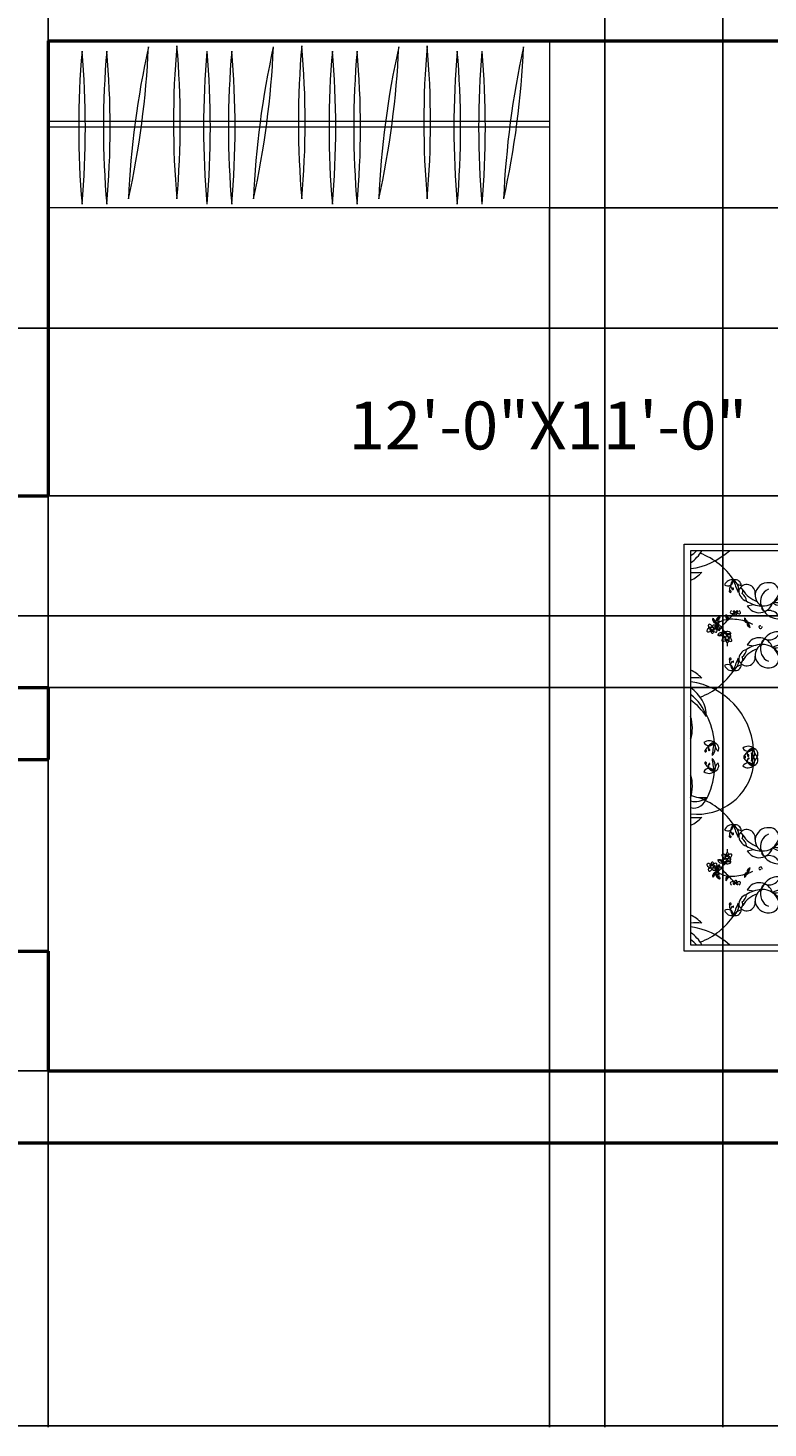
# Model space of a CAD drawing. Units: inches. Extents: x 3 to 576, y -689 to 51.
# Tile 2 of 21: x 109 to 201, y -689 to -514. Entities that reach past the tile are written whole.
import ezdxf

# ---------------------------------------------------------------- set-up
doc = ezdxf.new("R2010")
doc.units = ezdxf.units.IN
doc.header["$MEASUREMENT"] = 0
for name, color, linetype, lineweight in [('A-ANNO-DIMS', 2, 'Continuous', 18), ('A-AREA-IDEN', 7, 'Continuous', 18), ('A-FURN', 8, 'Continuous', 18), ('A-WALL', 7, 'Continuous', 50)]:
    doc.layers.add(name, color=color, linetype=linetype, lineweight=lineweight)
doc.styles.get("Standard").update_dxf_attribs({"font": 'arial.ttf'})
doc.dimstyles.get("Standard").update_dxf_attribs({"dimtxt": 0.18, "dimasz": 0.18, "dimexe": 0.18, "dimexo": 0.0625, "dimgap": 0.09, "dimtad": 0, "dimtih": 1, "dimtoh": 1, "dimdec": 0, "dimzin": 0, "dimdsep": 46, "dimlunit": 3, "dimtxsty": 'Standard', "dimcen": 0.09, "dimadec": 0, "dimazin": 0, "dimtfac": 1, "dimtdec": 0, "dimtofl": 0, "dimtmove": 0, "dimatfit": 3, "dimfxl": 1, "dimtolj": 1, "dimtzin": 0, "dimarcsym": 0})

# ---------------------------------------------------------------- blocks, each defined once
blk = doc.blocks.new('BED-DOUBLE')
for p, q in [((59.45, 69.91), (59.45, 0)), ((53.63, 58.35), (53.63, 67.49)), ((49.06, 62.92), (58.2, 62.92)), ((0, 60.68), (25.18, 60.68)), ((0, 9.72), (0, 60.68)), ((0.81, 59.87), (0.81, 10.53)), ((24.37, 59.87), (0.81, 59.87)), ((24.37, 56.73), (24.37, 59.87)), ((25.18, 60.68), (25.18, 56.73)), ((19.95, 13.6), (19.95, 56.73)), ((20.82, 13.66), (20.82, 56.73)), ((38.97, 55.99), (39.54, 56.55)), ((39.54, 56.55), (42.51, 54.01)), ((39.25, 53.16), (38.97, 55.99)), ((59.45, 55.93), (40.27, 55.93)), ((48.41, 55.93), (48.41, 13.98)), ((58.56, 13.98), (58.56, 55.93)), ((7.9, 52.98), (8.69, 53.14)), ((38.97, 49.62), (39.25, 53.16)), ((42.51, 54.01), (44.49, 51.31)), ((44.49, 51.31), (46.33, 46.22)), ((13.08, 20.76), (13.08, 49.15)), ((38.55, 46.5), (38.97, 49.62)), ((7.9, 48.1), (8.69, 47.94)), ((37.7, 44.66), (38.55, 46.5)), ((46.33, 46.22), (48.41, 38.59)), ((37.13, 42.39), (37.7, 44.66)), ((38.97, 42.11), (37.13, 42.39)), ((43.07, 40.55), (38.97, 42.11)), ((41.87, 14.23), (41.76, 41.05)), ((42.58, 14.23), (42.48, 40.78)), ((48.41, 36.72), (43.07, 40.55)), ((44.78, 14.2), (44.43, 39.58)), ((45.5, 14.17), (45.15, 39.06)), ((7.9, 22.3), (8.69, 22.46)), ((7.9, 17.41), (8.69, 17.26)), ((24.37, 10.53), (24.37, 13.61)), ((25.18, 13.59), (25.18, 9.72)), ((0.81, 10.53), (24.37, 10.53)), ((53.63, 11.56), (53.63, 2.42)), ((25.18, 9.72), (0, 9.72)), ((49.06, 6.99), (58.2, 6.99))]:
    blk.add_line(p, q)
for points in [[(47.8, 55.93), (47.8, 69.91), (59.45, 69.91)], [(53.63, 62.92), (52.22, 62.1)], [(53.63, 62.92), (55.04, 62.1)], [(59.45, 13.98), (47.8, 13.98), (47.8, 0), (59.45, 0)], [(53.63, 6.99), (52.22, 7.81)], [(53.63, 6.99), (55.04, 7.81)]]:
    blk.add_lwpolyline(points)
for points in [[(33.13, 56.7, 0.001242), (19.87, 56.73, -0.127202), (13.26, 58.14)], [(57.71, 51.91, 0.074897), (53.14, 51.83, -0.472817)], [(52.89, 35.28, 0.14099), (57.55, 35.14, 0.235245)], [(52.89, 32.3, -0.14099), (57.55, 32.44, -0.235245)], [(57.71, 18, -0.074897), (53.14, 18.08, 0.472817)], [(21.37, 13.68, 0.056112), (17.53, 13.18, 0.095341), (13.82, 12.19)]]:
    blk.add_lwpolyline(points, format="xyb")
for centre, radius in [((53.63, 62.92), 3.26), ((53.63, 62.92), 1.63), ((3.49, 50.11), 0.178), ((5.36, 48.94), 0.178), ((5.36, 21.45), 0.178), ((3.49, 20.29), 0.178), ((53.63, 6.99), 3.26), ((53.63, 6.99), 1.63)]:
    blk.add_circle(centre, radius)
for centre, radius, start, end in [((-2.47, 63.69), 5.54, 306.3036, 316.4814), ((-1.64, 62.09), 4.45, 303.4617, 330.1116), ((-0.42, 66.67), 9.13, 277.745, 311.8856), ((-1.32, 51.05), 9.13, 34.3865, 68.5908), ((13.3, 57.49), 0.645, 93.98, 207.3412), ((-0.61, 59.6), 3.71, 292.5547, 318.9546), ((1.38, 69.77), 12.63, 267.4081, 273.6519), ((6, 55.22), 1.01, 77.7115, 159.0387), ((5.45, 56.23), 0.762, 238.4633, 358.2869), ((7.95, 54.69), 2.31, 138.8402, 177.9352), ((6.56, 55.55), 0.747, 117.6827, 223.7762), ((6.39, 55.47), 0.757, 2.9516, 103.728), ((12.45, 57.59), 6.39, 192.5173, 207.1824), ((5.37, 55.04), 1.44, 345.4653, 54.2343), ((7.54, 57.02), 1.56, 211.3827, 255.2969), ((-59.69, 49.98), 72.78, 359.3433, 5.6887), ((37.8, 120.65), 64.12, 265.8294, 271.553), ((64.29, 55.36), 26.39, 177.4519, 191.3392), ((5.76, 54.77), 0.113, 177.9352, 11.4834), ((5.81, 54.78), 0.0551, 11.4834, 127.9409), ((6.09, 55.1), 0.0988, 223.7762, 159.7183), ((7.84, 54.58), 1.05, 350.264, 160.8688), ((8.16, 54.83), 1.31, 175.969, 254.3045), ((6.7, 54.8), 0.643, 333.9755, 53.2681), ((6.41, 53.42), 1.4, 6.1662, 51.5825), ((10.15, 56.66), 3.3, 211.2614, 251.7045), ((10.53, 54.2), 1.67, 84.9449, 172.8857), ((10.9, 54.49), 2.03, 182.3591, 234.0401), ((11.17, 53.54), 1.62, 111.5819, 201.4221), ((9.83, 55.04), 2.1, 265.2933, 346.921), ((10.7, 54.68), 1.18, 354.4856, 91.0538), ((8.16, 57.76), 5.29, 303.6671, 333.2997), ((9.88, 56.69), 3.75, 236.2883, 266.5076), ((9.4, 53.85), 1.74, 209.9085, 343.1337), ((10.13, 52.75), 0.434, 167.3041, 285.1471), ((11.31, 50.67), 2.7, 122.7011, 126.3445), ((11.81, 53.58), 2.23, 199.2822, 299.1751), ((12.57, 55.82), 2.9, 238.8218, 279.1554), ((11.31, 50.67), 2.7, 55.785, 94.7304), ((12.31, 52.24), 0.842, 30.0293, 52.325), ((3.75, 51.26), 0.199, 124.3538, 214.3923), ((4.04, 51.23), 0.464, 190.3057, 287.1958), ((4.17, 51.39), 0.538, 176.9701, 248.2913), ((8.01, 54.23), 5.2, 212.6784, 216.3746), ((3.99, 51.27), 0.206, 216.3746, 291.7548), ((2.83, 48.01), 3.1, 63.7819, 68.2913), ((4.48, 51.12), 0.464, 122.8155, 187.3992), ((4.12, 50.93), 0.155, 289.3605, 111.7548), ((4.24, 50.93), 0.155, 221.8703, 44.2646), ((4.69, 51.06), 0.538, 109.4799, 177.6828), ((4.4, 51.4), 0.199, 56.8636, 146.9021), ((4.5, 51.18), 0.206, 148.8844, 224.2646), ((8.78, 48.6), 5.2, 145.1882, 148.8844), ((5.81, 48.38), 2.9, 94.756, 119.2041), ((11.99, 44.2), 9.55, 132.2412, 142.1744), ((7.17, 51.8), 1.97, 178.3264, 187.1302), ((5.04, 51.53), 0.367, 11.3256, 64.4621), ((6.29, 52.06), 1.1, 190.2588, 210.656), ((5.55, 51.61), 0.336, 188.3432, 274.2869), ((5.84, 51.79), 0.586, 210.656, 242.6341), ((6.28, 52.3), 1.12, 218.2101, 226.3071), ((5.45, 51.35), 0.142, 325.7657, 67.4417), ((1.03, 56.11), 6.64, 313.1541, 322.0459), ((5.96, 45.49), 5.79, 73.5842, 93.8277), ((5.91, 52.13), 0.137, 142.4737, 265.053), ((6.09, 52.15), 0.294, 127.7621, 169.0403), ((5.94, 52.4), 0.414, 265.053, 338.3618), ((6.48, 51.84), 0.541, 113.4276, 137.6104), ((6.42, 52.4), 0.178, 183.2768, 356.7232), ((6.55, 52.07), 0.291, 139.7889, 227.6792), ((6.46, 51.97), 0.153, 227.6792, 350.3487), ((5.87, 52.08), 0.583, 353.0852, 15.7171), ((6.25, 52.01), 0.368, 350.3487, 43.6538), ((6.93, 52.39), 0.428, 198.7263, 262.5032), ((6.59, 52.19), 0.17, 1.1081, 91.8675), ((6.91, 52.1), 0.138, 255.2356, 54.9248), ((6.7, 52.15), 0.297, 11.5637, 52.6358), ((9.52, 51.39), 1.97, 178.3264, 187.1302), ((7.39, 51.11), 0.367, 11.3256, 64.4621), ((8.64, 51.64), 1.1, 190.2588, 210.656), ((7.9, 51.19), 0.336, 188.3432, 274.2869), ((8.19, 51.38), 0.586, 210.656, 242.6341), ((8.64, 51.88), 1.12, 218.2101, 226.3071), ((7.81, 50.93), 0.142, 325.7657, 67.4417), ((8.21, 50.67), 0.336, 147.5332, 233.4768), ((7.94, 50.71), 0.142, 354.3784, 96.0543), ((8.51, 50.85), 0.586, 179.1859, 211.164), ((5.96, 45.49), 5.79, 63.0032, 69.8941), ((10.62, 50.95), 1.43, 41.5653, 105.1471), ((11.41, 53.92), 2.01, 277.436, 299.9149), ((12.48, 52.59), 1.05, 221.5653, 293.8354), ((12.31, 52.24), 0.842, 314.4517, 333.558), ((58.53, 49.42), 9.37, 165.1039, 191.0369), ((51.31, 43.01), 9.01, 65.1316, 101.7583), ((723.03, 13.38), 666.43, 176.68521, 177.14978), ((2.98, 49.84), 0.137, 142.4737, 265.053), ((3.16, 49.87), 0.294, 61.2196, 169.0403), ((3, 50.12), 0.414, 265.053, 338.3618), ((3.35, 50.47), 0.351, 157.4086, 261.4386), ((3.15, 50.48), 0.176, 58.0499, 135.6268), ((3.55, 49.55), 0.541, 113.4276, 137.6104), ((3.34, 50.37), 0.118, 172.906, 277.132), ((2.95, 50.16), 0.561, 14.7558, 58.0499), ((3.62, 49.79), 0.291, 139.7889, 227.6792), ((3.53, 49.68), 0.153, 227.6792, 350.3487), ((3.74, 50.31), 0.243, 36.1046, 181.4281), ((2.93, 49.79), 0.583, 353.0852, 15.7171), ((3.31, 49.72), 0.368, 350.3487, 43.6538), ((3.59, 50.5), 0.245, 270.0645, 331.1507), ((3.8, 50.44), 0.28, 221.8413, 265.7877), ((4, 50.1), 0.428, 198.7263, 262.5032), ((3.66, 49.9), 0.17, 1.1081, 91.8675), ((3.8, 50.33), 0.174, 263.7526, 41.7054), ((3.76, 49.86), 0.297, 11.5637, 86.365), ((5.81, 48.38), 2.9, 124.0033, 132.4917), ((3.98, 49.81), 0.138, 255.2356, 54.9248), ((4.48, 50.4), 0.493, 128.3208, 208.8162), ((4.57, 50.43), 0.59, 207.7043, 254.3516), ((4.94, 50.48), 0.812, 157.2305, 229.0635), ((4.67, 50.75), 0.478, 174.4544, 220.6188), ((4.19, 50.1), 0.812, 270.278, 342.111), ((4.73, 49.08), 0.574, 98.7227, 159.3375), ((4.44, 49.82), 0.59, 244.9899, 291.6373), ((1.96, 48.08), 3.48, 30.544, 49.818), ((3.87, 50.06), 0.574, 340.0041, 40.6188), ((4.57, 50.12), 0.478, 278.7227, 324.8872), ((4.49, 49.73), 0.493, 290.5253, 358.5375), ((5.23, 49.31), 0.351, 157.4086, 261.4386), ((5.03, 49.32), 0.176, 58.0499, 135.6268), ((5.45, 49.87), 0.493, 182.8499, 266.1226), ((5.26, 50.22), 0.478, 231.7607, 277.9252), ((5.63, 50.31), 0.812, 214.5369, 286.3699), ((5.21, 49.21), 0.118, 172.906, 277.132), ((4.83, 48.99), 0.561, 14.7558, 58.0499), ((1.96, 48.08), 3.48, 23.0501, 23.8477), ((5.4, 49.18), 0.574, 37.3105, 97.9252), ((5.61, 49.14), 0.243, 36.1046, 181.4281), ((5.47, 49.97), 0.59, 265.0106, 311.658), ((5.47, 49.33), 0.245, 270.0645, 331.1507), ((5.68, 49.17), 0.174, 263.7526, 41.7054), ((8.95, 51.12), 1.1, 211.164, 231.5612), ((9.15, 52.01), 1.97, 234.6898, 243.4936), ((9.16, 51), 1.12, 195.5129, 203.6099), ((7.9, 50.27), 0.367, 357.3579, 50.4944), ((9.48, 50.34), 0.135, 12.7051, 190.4384), ((9.56, 50.36), 0.219, 190.4384, 10.4136), ((11.81, 47.5), 2.23, 60.8249, 160.7178), ((10.62, 50.13), 1.43, 254.8529, 318.4347), ((11.41, 47.16), 2.01, 60.0851, 82.564), ((12.48, 48.49), 1.05, 66.1646, 138.4347), ((12.31, 48.84), 0.842, 23.229, 45.5483), ((32.84, 49.05), 5.69, 336.2616, 11.3392), ((4.85, 48.67), 0.137, 142.4737, 265.053), ((5.03, 48.7), 0.294, 61.2196, 169.0403), ((4.88, 48.95), 0.414, 265.053, 338.3618), ((5.43, 48.38), 0.541, 113.4276, 137.6104), ((5.5, 48.62), 0.291, 139.7889, 227.6792), ((5.4, 48.52), 0.153, 227.6792, 350.3487), ((4.81, 48.63), 0.583, 353.0852, 15.7171), ((1.96, 48.08), 3.48, 357.1071, 4.7585), ((5.19, 48.56), 0.368, 350.3487, 43.6538), ((5.68, 49.27), 0.28, 221.8413, 265.7877), ((5.87, 48.94), 0.428, 198.7263, 262.5032), ((5.53, 48.74), 0.17, 1.1081, 91.8675), ((5.64, 48.7), 0.297, 11.5637, 86.365), ((5.85, 48.65), 0.138, 255.2356, 54.9248), ((8.16, 46.25), 1.31, 105.6955, 184.031), ((6.41, 47.66), 1.4, 308.4175, 353.8338), ((10.15, 44.42), 3.3, 108.2955, 148.7386), ((9.88, 44.39), 3.75, 93.4924, 123.7117), ((9.4, 47.23), 1.74, 16.8663, 150.0915), ((10.9, 46.59), 2.03, 125.9599, 177.6409), ((11.17, 47.54), 1.62, 158.5779, 248.4181), ((9.83, 46.04), 2.1, 13.079, 94.7067), ((10.13, 48.33), 0.434, 74.8529, 192.6959), ((11.31, 50.41), 2.7, 233.6555, 237.2989), ((12.57, 45.26), 2.9, 79.7133, 121.1782), ((11.31, 50.41), 2.7, 265.2696, 304.215), ((8.16, 43.32), 5.29, 21.4941, 56.3329), ((12.31, 48.84), 0.842, 307.675, 336.7144), ((65.19, 44.49), 16.25, 168.0397, 199.2615), ((5.45, 44.85), 0.762, 1.7131, 121.5367), ((5.76, 46.31), 0.113, 348.5166, 182.0648), ((7.95, 46.39), 2.31, 182.0648, 221.1598), ((5.81, 46.3), 0.0551, 232.0591, 348.5166), ((6.56, 45.54), 0.747, 136.2238, 242.3173), ((6.13, 45.97), 0.0595, 200.2667, 136.2271), ((5.37, 46.05), 1.44, 305.7657, 14.5347), ((12.45, 43.49), 6.39, 152.8176, 167.4827), ((7.84, 46.5), 1.05, 199.1312, 9.736), ((6.7, 46.28), 0.643, 306.7319, 26.0245), ((10.53, 46.88), 1.67, 187.1143, 275.0551), ((10.7, 46.4), 1.18, 268.9462, 5.5144), ((63.55, 37.54), 27.11, 160.1194, 169.3383), ((32.41, 42.33), 25.35, 352.2196, 9.497), ((-0.61, 41.48), 3.71, 41.0454, 67.4453), ((1.38, 31.32), 12.63, 86.3481, 92.5919), ((-1.32, 50.03), 9.13, 291.4092, 325.6135), ((6, 45.86), 1.01, 200.9613, 282.2885), ((6.39, 45.61), 0.757, 256.272, 357.0484), ((7.54, 44.06), 1.56, 104.7031, 148.6173), ((-0.42, 34.41), 9.13, 4.4623, 82.255), ((-1.64, 38.99), 4.45, 1.272, 56.5383), ((37.07, 42.55), 0.169, 178.8623, 289.7536), ((-2.47, 37.39), 5.54, 17.8504, 53.6964), ((-4.03, 34.48), 8.25, 34.0123, 54.053), ((-3.99, 37.66), 5.02, 343.5431, 17.0202), ((-5.31, 35.11), 9.13, 4.4623, 27.4146), ((61.64, 37.91), 12.33, 169.8617, 193.6238), ((45.23, 36.98), 12.46, 351.5249, 13.96), ((-6.58, 35.67), 7.42, 4.3787, 5.6357), ((-11.66, 31.77), 13.27, 19.7217, 19.9028), ((3.11, 35.07), 1.01, 47.7873, 129.1145), ((3.14, 36.22), 0.762, 208.5391, 328.3627), ((4.54, 33.64), 2.31, 108.9159, 148.011), ((3.76, 35.07), 0.747, 87.7585, 193.852), ((9.89, 33.91), 6.39, 162.593, 177.2582), ((2.48, 35.23), 1.44, 315.5411, 24.3101), ((5.35, 35.86), 1.56, 181.4585, 225.3727), ((3.58, 35.09), 0.757, 333.0274, 73.8037), ((8, 34.37), 1.01, 47.7873, 129.1145), ((8.03, 35.52), 0.762, 208.5391, 328.3627), ((9.43, 32.94), 2.31, 108.9159, 148.011), ((8.65, 34.38), 0.747, 87.7585, 193.852), ((7.37, 34.53), 1.44, 315.5411, 24.3101), ((14.78, 33.21), 6.39, 162.593, 177.2582), ((8.47, 34.4), 0.757, 333.0274, 73.8037), ((10.24, 35.16), 1.56, 181.4585, 225.3727), ((50.55, 43.52), 8.57, 264.0129, 285.8293), ((2.68, 34.8), 0.113, 148.011, 341.5592), ((2.68, 33.27), 0.113, 18.4408, 211.989), ((2.73, 34.78), 0.0551, 341.5592, 98.0167), ((3.13, 34.92), 0.0988, 193.852, 129.9245), ((9.89, 34.16), 6.39, 182.7418, 197.407), ((2.48, 32.84), 1.44, 335.6899, 44.4589), ((5.35, 32.21), 1.56, 134.6273, 178.5415), ((3.58, 32.97), 0.757, 286.1963, 26.9726), ((7.57, 34.1), 0.113, 148.011, 341.5592), ((7.57, 33.97), 0.113, 18.4408, 211.989), ((9.43, 35.13), 2.31, 211.989, 251.0841), ((7.62, 34.08), 0.0551, 341.5592, 98.0167), ((7.62, 33.99), 0.0551, 261.9833, 18.4408), ((8.65, 33.69), 0.747, 166.148, 272.2415), ((8.02, 34.22), 0.0988, 193.852, 129.9245), ((8.06, 33.86), 0.0595, 230.1909, 166.0209), ((7.37, 33.54), 1.44, 335.6899, 44.4589), ((14.78, 34.86), 6.39, 182.7418, 197.407), ((8.47, 33.67), 0.757, 286.1963, 26.9726), ((10.24, 32.91), 1.56, 134.6273, 178.5415), ((1.69, 33.95), 7.07, 262.8636, 351.8197), ((-3.99, 30.4), 5.02, 342.9798, 16.4569), ((-6.58, 32.39), 7.42, 354.3643, 355.6213), ((-11.66, 36.3), 13.27, 340.0972, 340.2783), ((3.14, 31.85), 0.762, 31.6373, 151.4609), ((3.11, 33), 1.01, 230.8855, 312.2127), ((4.54, 34.43), 2.31, 211.989, 251.0841), ((2.73, 33.29), 0.0551, 261.9833, 18.4408), ((-5.31, 32.96), 9.13, 332.5854, 355.5377), ((3.76, 32.99), 0.747, 166.148, 272.2415), ((3.17, 33.16), 0.0595, 230.1909, 166.0209), ((8.03, 32.55), 0.762, 31.6373, 151.4609), ((8, 33.7), 1.01, 230.8855, 312.2127), ((53.02, 31.01), 3.71, 155.0183, 198.5407), ((50.55, 24.06), 8.57, 74.1707, 95.9871), ((54.23, 31.48), 3.46, 333.3437, 16.1026), ((2.33, 33.04), 4.09, 248.117, 276.6195), ((1.2, 29.29), 1.64, 256.3898, 349.0739), ((1.42, 30.52), 2.07, 252.8609, 311.9049), ((-1.32, 20.37), 9.13, 34.3865, 68.5908), ((57.84, 24.53), 8.9, 153.8761, 196.1746), ((45.48, 26.29), 12.29, 346.3427, 11.1841), ((1.38, 39.08), 12.63, 267.4081, 273.6519), ((-0.61, 28.92), 3.71, 292.5547, 318.9546), ((6, 24.53), 1.01, 77.7115, 159.0387), ((5.45, 25.55), 0.762, 238.4633, 358.2869), ((7.95, 24), 2.31, 138.8402, 177.9352), ((6.56, 24.86), 0.747, 117.6827, 223.7762), ((6.39, 24.79), 0.757, 2.9516, 103.728), ((7.54, 26.34), 1.56, 211.3827, 255.2969), ((5.37, 24.35), 1.44, 345.4653, 54.2343), ((12.45, 26.91), 6.39, 192.5173, 207.1824), ((7.84, 23.9), 1.05, 350.264, 160.8688), ((6.7, 24.12), 0.643, 333.9755, 53.2681), ((10.53, 23.52), 1.67, 84.9449, 172.8857), ((10.7, 24), 1.18, 354.4856, 91.0538), ((8.16, 27.08), 5.29, 303.6671, 338.5059), ((5.76, 24.08), 0.113, 177.9352, 11.4834), ((5.81, 24.09), 0.0551, 11.4834, 127.9409), ((6.09, 24.41), 0.0988, 223.7762, 159.7183), ((8.16, 24.15), 1.31, 175.969, 254.3045), ((6.41, 22.74), 1.4, 6.1662, 51.5825), ((10.15, 25.98), 3.3, 211.2614, 251.7045), ((9.88, 26.01), 3.75, 236.2883, 266.5076), ((10.9, 23.81), 2.03, 182.3591, 234.0401), ((11.17, 22.86), 1.62, 111.5819, 201.4221), ((9.83, 24.36), 2.1, 265.2933, 346.921), ((723.03, 56.53), 666.43, 182.85022, 183.31479), ((4.44, 20.58), 0.59, 68.3627, 115.0101), ((4.19, 20.3), 0.812, 17.889, 89.722), ((4.73, 21.32), 0.574, 200.6625, 261.2773), ((4.49, 20.66), 0.493, 1.4625, 69.4747), ((4.85, 21.72), 0.137, 94.947, 217.5263), ((5.03, 21.7), 0.294, 190.9597, 298.7804), ((4.88, 21.45), 0.414, 21.6382, 94.947), ((5.23, 21.09), 0.351, 98.5614, 202.5914), ((5.43, 22.01), 0.541, 222.3896, 246.5724), ((5.21, 21.19), 0.118, 82.868, 187.094), ((4.83, 21.41), 0.561, 301.9501, 345.2442), ((5.5, 21.78), 0.291, 132.3208, 220.2111), ((5.4, 21.88), 0.153, 9.6513, 132.3208), ((4.81, 21.77), 0.583, 344.2829, 6.9148), ((5.61, 21.26), 0.243, 178.5719, 323.8954), ((1.96, 22.32), 3.48, 355.2415, 2.8929), ((5.19, 21.84), 0.368, 316.3462, 9.6513), ((5.87, 21.46), 0.428, 97.4968, 161.2737), ((5.68, 21.12), 0.28, 94.2123, 138.1587), ((5.47, 21.07), 0.245, 28.8493, 89.9355), ((5.53, 21.66), 0.17, 268.1325, 358.8919), ((5.64, 21.7), 0.297, 273.635, 348.4363), ((5.68, 21.23), 0.174, 318.2946, 96.2474), ((5.85, 21.75), 0.138, 305.0752, 104.7644), ((9.4, 23.17), 1.74, 209.9085, 343.1337), ((10.13, 22.07), 0.434, 167.3041, 285.1471), ((11.31, 19.99), 2.7, 122.7011, 126.3445), ((11.81, 22.9), 2.23, 199.2822, 299.1751), ((10.62, 20.26), 1.43, 41.5653, 105.1471), ((12.57, 25.14), 2.9, 238.8218, 280.2867), ((11.31, 19.99), 2.7, 55.785, 94.7304), ((11.41, 23.23), 2.01, 277.436, 299.9149), ((12.48, 21.91), 1.05, 221.5653, 293.8354), ((12.31, 21.55), 0.842, 23.2856, 52.325), ((12.31, 21.55), 0.842, 314.4517, 336.7144), ((58.53, 20.49), 9.37, 168.9631, 194.8961), ((2.98, 20.56), 0.137, 94.947, 217.5263), ((3.16, 20.53), 0.294, 190.9597, 298.7804), ((3, 20.28), 0.414, 21.6382, 94.947), ((3.35, 19.93), 0.351, 98.5614, 202.5914), ((3.15, 19.91), 0.176, 224.3732, 301.9501), ((3.55, 20.85), 0.541, 222.3896, 246.5724), ((3.34, 20.03), 0.118, 82.868, 187.094), ((2.95, 20.24), 0.561, 301.9501, 345.2442), ((3.62, 20.61), 0.291, 132.3208, 220.2111), ((3.53, 20.71), 0.153, 9.6513, 132.3208), ((2.93, 20.61), 0.583, 344.2829, 6.9148), ((3.74, 20.09), 0.243, 178.5719, 323.8954), ((3.31, 20.68), 0.368, 316.3462, 9.6513), ((4.04, 19.17), 0.464, 72.8042, 169.6943), ((4, 20.3), 0.428, 97.4968, 161.2737), ((3.8, 19.96), 0.28, 94.2123, 138.1587), ((3.59, 19.9), 0.245, 28.8493, 89.9355), ((4.17, 19.01), 0.538, 111.7087, 183.0299), ((3.66, 20.5), 0.17, 268.1325, 358.8919), ((3.76, 20.54), 0.297, 273.635, 348.4363), ((3.8, 20.07), 0.174, 318.2946, 96.2474), ((3.99, 19.13), 0.206, 68.2452, 143.6254), ((5.81, 22.02), 2.9, 227.5083, 235.9967), ((3.98, 20.59), 0.138, 305.0752, 104.7644), ((2.83, 22.39), 3.1, 291.7087, 296.2181), ((4.48, 20), 0.493, 151.1838, 231.6792), ((4.48, 19.27), 0.464, 172.6008, 237.1845), ((4.57, 19.96), 0.59, 105.6484, 152.2957), ((4.12, 19.47), 0.155, 248.2452, 70.6395), ((4.94, 19.92), 0.812, 130.9365, 202.7695), ((4.24, 19.47), 0.155, 315.7354, 138.1297), ((4.69, 19.33), 0.538, 182.3172, 250.5201), ((4.67, 19.65), 0.478, 139.3812, 185.5456), ((1.96, 22.32), 3.48, 310.182, 329.456), ((4.5, 19.21), 0.206, 135.7354, 211.1156), ((3.87, 20.33), 0.574, 319.3812, 19.9959), ((5.81, 22.02), 2.9, 240.7959, 265.244), ((11.99, 26.2), 9.55, 217.8256, 227.7588), ((4.57, 20.28), 0.478, 35.1128, 81.2773), ((5.03, 21.08), 0.176, 224.3732, 301.9501), ((5.45, 20.52), 0.493, 93.8774, 177.1501), ((5.63, 20.09), 0.812, 73.6301, 145.4631), ((5.26, 20.18), 0.478, 82.0748, 128.2393), ((1.96, 22.32), 3.48, 336.1523, 336.9499), ((5.4, 21.22), 0.574, 262.0748, 322.6895), ((5.47, 20.43), 0.59, 48.342, 94.9894), ((5.96, 24.9), 5.79, 266.1723, 286.4158), ((8.64, 18.76), 1.1, 149.344, 169.7412), ((7.9, 19.21), 0.336, 85.7131, 171.6568), ((8.19, 19.02), 0.586, 117.3659, 149.344), ((8.64, 18.52), 1.12, 133.6929, 141.7899), ((7.81, 19.46), 0.142, 292.5583, 34.2343), ((8.21, 19.72), 0.336, 126.5232, 212.4668), ((8.51, 19.55), 0.586, 148.836, 180.8141), ((7.94, 19.68), 0.142, 263.9457, 5.6216), ((5.96, 24.9), 5.79, 290.1059, 296.9968), ((8.95, 19.28), 1.1, 128.4388, 148.836), ((9.15, 18.38), 1.97, 116.5064, 125.3102), ((9.16, 19.4), 1.12, 156.3901, 164.4871), ((7.9, 20.13), 0.367, 309.5056, 2.6421), ((9.56, 20.04), 0.219, 349.5864, 169.5616), ((9.48, 20.06), 0.135, 169.5616, 347.2949), ((-54.91, 18.62), 68.03, 355.2402, 1.8035), ((3.75, 19.14), 0.199, 145.6077, 235.6462), ((8.01, 16.17), 5.2, 143.6254, 147.3216), ((4.4, 18.99), 0.199, 213.0979, 303.1364), ((8.78, 21.8), 5.2, 211.1156, 214.8118), ((6.29, 18.34), 1.1, 149.344, 169.7412), ((7.17, 18.6), 1.97, 172.8698, 181.6736), ((5.04, 18.87), 0.367, 295.5379, 348.6744), ((5.55, 18.79), 0.336, 85.7131, 171.6568), ((5.84, 18.61), 0.586, 117.3659, 149.344), ((6.28, 18.1), 1.12, 133.6929, 141.7899), ((5.45, 19.05), 0.142, 292.5583, 34.2343), ((1.03, 14.28), 6.64, 37.9541, 46.8459), ((5.91, 18.27), 0.137, 94.947, 217.5263), ((6.09, 18.24), 0.294, 190.9597, 232.2379), ((5.94, 18), 0.414, 21.6382, 94.947), ((6.48, 18.56), 0.541, 222.3896, 246.5724), ((6.42, 18), 0.178, 3.2768, 176.7232), ((6.55, 18.32), 0.291, 132.3208, 220.2111), ((6.46, 18.43), 0.153, 9.6513, 132.3208), ((5.87, 18.32), 0.583, 344.2829, 6.9148), ((6.25, 18.39), 0.368, 316.3462, 9.6513), ((6.93, 18.01), 0.428, 97.4968, 161.2737), ((6.59, 18.21), 0.17, 268.1325, 358.8919), ((6.91, 18.3), 0.138, 305.0752, 104.7644), ((6.7, 18.25), 0.297, 307.3642, 348.4363), ((9.52, 19.01), 1.97, 172.8698, 181.6736), ((7.39, 19.29), 0.367, 295.5379, 348.6744), ((9.4, 16.55), 1.74, 16.8663, 150.0915), ((10.9, 15.91), 2.03, 125.9599, 177.6409), ((10.13, 17.65), 0.434, 74.8529, 192.6959), ((11.81, 16.82), 2.23, 60.8249, 160.7178), ((11.31, 19.72), 2.7, 233.6555, 237.2989), ((10.62, 19.45), 1.43, 254.8529, 318.4347), ((11.41, 16.48), 2.01, 60.0851, 82.564), ((12.48, 17.81), 1.05, 66.1646, 138.4347), ((12.31, 18.16), 0.842, 307.675, 342.5814), ((12.31, 18.16), 0.842, 16.6343, 45.5483), ((51.31, 26.9), 9.01, 258.2417, 294.8684), ((8.16, 15.56), 1.31, 105.6955, 184.031), ((7.84, 15.82), 1.05, 199.1312, 9.736), ((6.7, 15.6), 0.643, 306.7319, 26.0245), ((6.41, 16.98), 1.4, 308.4175, 353.8338), ((10.15, 13.74), 3.3, 108.2955, 148.7386), ((9.88, 13.7), 3.75, 93.4924, 123.7117), ((10.53, 16.2), 1.67, 187.1143, 275.0551), ((11.17, 16.86), 1.62, 158.5779, 248.4181), ((9.83, 15.35), 2.1, 13.079, 94.7067), ((10.7, 15.72), 1.18, 268.9462, 5.5144), ((12.57, 14.57), 2.9, 79.249, 121.1782), ((11.31, 19.72), 2.7, 265.2696, 304.215), ((8.16, 12.63), 5.29, 23.6453, 56.3329), ((-0.61, 10.8), 3.71, 41.0454, 67.4453), ((-1.32, 19.35), 9.13, 291.4092, 325.6135), ((5.45, 14.17), 0.762, 1.7131, 121.5367), ((6, 15.18), 1.01, 200.9613, 282.2885), ((5.76, 15.63), 0.113, 348.5166, 182.0648), ((7.95, 15.71), 2.31, 182.0648, 221.1598), ((5.81, 15.62), 0.0551, 232.0591, 348.5166), ((6.56, 14.85), 0.747, 136.2238, 242.3173), ((6.13, 15.29), 0.0595, 200.2667, 136.2271), ((12.45, 12.81), 6.39, 152.8176, 167.4827), ((5.37, 15.36), 1.44, 305.7657, 14.5347), ((7.54, 13.38), 1.56, 104.7031, 148.6173), ((6.39, 14.93), 0.757, 256.272, 357.0484), ((35.29, -149.59), 163.86, 89.1145, 94.8735), ((39.86, -111.34), 125.62, 86.1, 90.9282), ((1.38, 0.63), 12.63, 86.3481, 92.5919), ((-0.42, 3.73), 9.13, 48.1144, 82.255), ((13.47, 12.72), 0.637, 156.5219, 303.8264), ((-1.64, 8.31), 4.45, 29.8884, 56.5383), ((-2.47, 6.71), 5.54, 43.5186, 53.6964)]:
    blk.add_arc(centre, radius, start, end)
blk = doc.blocks.new('*D50')
at = {"layer": 'A-ANNO-DIMS', "color": 0, "lineweight": -2, "transparency": 16777216}
for p, q in [((388.02, -644.37), (388.02, -688.94)), ((102.29, -653.37), (102.29, -688.94)), ((102.47, -688.76), (244.55, -688.76)), ((387.84, -688.76), (245.77, -688.76))]:
    blk.add_line(p, q, dxfattribs=at)
at = {"layer": 'A-ANNO-DIMS', "color": 0, "transparency": 16777216}
for points in [[(102.47, -688.73), (102.47, -688.79), (102.29, -688.76)], [(387.84, -688.73), (387.84, -688.79), (388.02, -688.76)]]:
    blk.add_solid(points, dxfattribs=at)
at = {"layer": 'Defpoints', "color": 0, "transparency": 16777216}
for p in [(388.02, -644.31), (102.29, -653.31), (388.02, -688.76)]:
    blk.add_point(p, dxfattribs=at)
at = {"layer": 'A-ANNO-DIMS', "color": 0, "transparency": 16777216, "insert": (245.16, -688.76), "char_height": 0.18, "attachment_point": 5}
blk.add_mtext('\\A1;23\'-9 1/2"', dxfattribs=at)
blk = doc.blocks.new('*D73')
at = {"layer": 'A-ANNO-DIMS', "color": 0, "lineweight": -2, "transparency": 16777216}
for p, q in [((531.23, -449.31), (2.66, -449.31)), ((2.84, -449.49), (2.84, -518.13)), ((2.84, -587.13), (2.84, -518.49)), ((531.23, -587.31), (2.66, -587.31))]:
    blk.add_line(p, q, dxfattribs=at)
at = {"layer": 'A-ANNO-DIMS', "color": 0, "transparency": 16777216}
for points in [[(2.81, -449.49), (2.87, -449.49), (2.84, -449.31)], [(2.81, -587.13), (2.87, -587.13), (2.84, -587.31)]]:
    blk.add_solid(points, dxfattribs=at)
at = {"layer": 'Defpoints', "color": 0, "transparency": 16777216}
for p in [(531.29, -449.31), (2.84, -587.31), (531.29, -587.31)]:
    blk.add_point(p, dxfattribs=at)
at = {"layer": 'A-ANNO-DIMS', "color": 0, "transparency": 16777216, "insert": (2.84, -518.31), "char_height": 0.18, "attachment_point": 5}
blk.add_mtext('\\A1;11\'-6"', dxfattribs=at)
blk = doc.blocks.new('*D74')
at = {"layer": 'A-ANNO-DIMS', "color": 0, "lineweight": -2, "transparency": 16777216}
for p, q in [((531.23, -587.31), (2.66, -587.31)), ((2.84, -587.49), (2.84, -591.63)), ((2.84, -596.13), (2.84, -591.99)), ((540.23, -596.31), (2.66, -596.31))]:
    blk.add_line(p, q, dxfattribs=at)
at = {"layer": 'A-ANNO-DIMS', "color": 0, "transparency": 16777216}
for points in [[(2.81, -587.49), (2.87, -587.49), (2.84, -587.31)], [(2.81, -596.13), (2.87, -596.13), (2.84, -596.31)]]:
    blk.add_solid(points, dxfattribs=at)
at = {"layer": 'Defpoints', "color": 0, "transparency": 16777216}
for p in [(531.29, -587.31), (2.84, -596.31), (540.29, -596.31)]:
    blk.add_point(p, dxfattribs=at)
at = {"layer": 'A-ANNO-DIMS', "color": 0, "transparency": 16777216, "insert": (2.84, -591.81), "char_height": 0.18, "attachment_point": 5}
blk.add_mtext('\\A1;0\'-9"', dxfattribs=at)
blk = doc.blocks.new('*D86')
at = {"layer": 'A-ANNO-DIMS', "color": 0, "lineweight": -2, "transparency": 16777216}
for p, q in [((111.29, -97.21), (111.29, -688.94)), ((195.78, -97.21), (195.78, -688.94)), ((111.47, -688.76), (153, -688.76)), ((195.6, -688.76), (154.08, -688.76))]:
    blk.add_line(p, q, dxfattribs=at)
at = {"layer": 'A-ANNO-DIMS', "color": 0, "transparency": 16777216}
for points in [[(111.47, -688.73), (111.47, -688.79), (111.29, -688.76)], [(195.6, -688.73), (195.6, -688.79), (195.78, -688.76)]]:
    blk.add_solid(points, dxfattribs=at)
at = {"layer": 'Defpoints', "color": 0, "transparency": 16777216}
for p in [(111.29, -97.15), (195.78, -97.15), (195.78, -688.76)]:
    blk.add_point(p, dxfattribs=at)
at = {"layer": 'A-ANNO-DIMS', "color": 0, "transparency": 16777216, "insert": (153.54, -688.76), "char_height": 0.18, "attachment_point": 5}
blk.add_mtext('\\A1;7\'-0 1/2"', dxfattribs=at)
blk = doc.blocks.new('*D90')
at = {"layer": 'A-ANNO-DIMS', "color": 0, "lineweight": -2, "transparency": 16777216}
for p, q in [((111.29, -409.62), (111.29, -688.94)), ((181.04, -409.62), (181.04, -688.94)), ((111.47, -688.76), (145.63, -688.76)), ((180.86, -688.76), (146.7, -688.76))]:
    blk.add_line(p, q, dxfattribs=at)
at = {"layer": 'A-ANNO-DIMS', "color": 0, "transparency": 16777216}
for points in [[(111.47, -688.73), (111.47, -688.79), (111.29, -688.76)], [(180.86, -688.73), (180.86, -688.79), (181.04, -688.76)]]:
    blk.add_solid(points, dxfattribs=at)
at = {"layer": 'Defpoints', "color": 0, "transparency": 16777216}
for p in [(111.29, -409.56), (181.04, -409.56), (181.04, -688.76)]:
    blk.add_point(p, dxfattribs=at)
at = {"layer": 'A-ANNO-DIMS', "color": 0, "transparency": 16777216, "insert": (146.17, -688.76), "char_height": 0.18, "attachment_point": 5}
blk.add_mtext('\\A1;5\'-9 1/2"', dxfattribs=at)
blk = doc.blocks.new('*D92')
at = {"layer": 'A-ANNO-DIMS', "color": 0, "lineweight": -2, "transparency": 16777216}
for p, q in [((111.29, -536.3), (111.29, -688.94)), ((174.08, -536.3), (174.08, -688.94)), ((111.47, -688.76), (142.36, -688.76)), ((173.9, -688.76), (143.02, -688.76))]:
    blk.add_line(p, q, dxfattribs=at)
at = {"layer": 'A-ANNO-DIMS', "color": 0, "transparency": 16777216}
for points in [[(111.47, -688.73), (111.47, -688.79), (111.29, -688.76)], [(173.9, -688.73), (173.9, -688.79), (174.08, -688.76)]]:
    blk.add_solid(points, dxfattribs=at)
at = {"layer": 'Defpoints', "color": 0, "transparency": 16777216}
for p in [(111.29, -536.24), (174.08, -536.24), (174.08, -688.76)]:
    blk.add_point(p, dxfattribs=at)
at = {"layer": 'A-ANNO-DIMS', "color": 0, "transparency": 16777216, "insert": (142.69, -688.76), "char_height": 0.18, "attachment_point": 5}
blk.add_mtext('\\A1;5\'-3"', dxfattribs=at)
blk = doc.blocks.new('*D93')
at = {"layer": 'A-ANNO-DIMS', "color": 0, "lineweight": -2, "transparency": 16777216}
for p, q in [((174.14, -515.31), (575.92, -515.31)), ((575.74, -515.49), (575.74, -525.59)), ((575.74, -536.06), (575.74, -525.96)), ((174.14, -536.24), (575.92, -536.24))]:
    blk.add_line(p, q, dxfattribs=at)
at = {"layer": 'A-ANNO-DIMS', "color": 0, "transparency": 16777216}
for points in [[(575.71, -515.49), (575.77, -515.49), (575.74, -515.31)], [(575.71, -536.06), (575.77, -536.06), (575.74, -536.24)]]:
    blk.add_solid(points, dxfattribs=at)
at = {"layer": 'Defpoints', "color": 0, "transparency": 16777216}
for p in [(174.08, -515.31), (174.08, -536.24), (575.74, -536.24)]:
    blk.add_point(p, dxfattribs=at)
at = {"layer": 'A-ANNO-DIMS', "color": 0, "transparency": 16777216, "insert": (575.74, -525.77), "char_height": 0.18, "attachment_point": 5}
blk.add_mtext('\\A1;1\'-9"', dxfattribs=at)
blk = doc.blocks.new('*D107')
at = {"layer": 'A-ANNO-DIMS', "color": 0, "lineweight": -2, "transparency": 16777216}
for p, q in [((111.36, -515.31), (575.92, -515.31)), ((575.74, -515.49), (575.74, -543.63)), ((575.74, -572.13), (575.74, -543.99)), ((111.36, -572.31), (575.92, -572.31))]:
    blk.add_line(p, q, dxfattribs=at)
at = {"layer": 'A-ANNO-DIMS', "color": 0, "transparency": 16777216}
for points in [[(575.71, -515.49), (575.77, -515.49), (575.74, -515.31)], [(575.71, -572.13), (575.77, -572.13), (575.74, -572.31)]]:
    blk.add_solid(points, dxfattribs=at)
at = {"layer": 'Defpoints', "color": 0, "transparency": 16777216}
for p in [(111.29, -515.31), (111.29, -572.31), (575.74, -572.31)]:
    blk.add_point(p, dxfattribs=at)
at = {"layer": 'A-ANNO-DIMS', "color": 0, "transparency": 16777216, "insert": (575.74, -543.81), "char_height": 0.18, "attachment_point": 5}
blk.add_mtext('\\A1;4\'-9"', dxfattribs=at)
blk = doc.blocks.new('*D109')
at = {"layer": 'A-ANNO-DIMS', "color": 0, "lineweight": -2, "transparency": 16777216}
for p, q in [((255.23, -551.31), (2.66, -551.31)), ((2.84, -551.49), (2.84, -597.63)), ((2.84, -644.13), (2.84, -597.99)), ((255.23, -644.31), (2.66, -644.31))]:
    blk.add_line(p, q, dxfattribs=at)
at = {"layer": 'A-ANNO-DIMS', "color": 0, "transparency": 16777216}
for points in [[(2.81, -551.49), (2.87, -551.49), (2.84, -551.31)], [(2.81, -644.13), (2.87, -644.13), (2.84, -644.31)]]:
    blk.add_solid(points, dxfattribs=at)
at = {"layer": 'Defpoints', "color": 0, "transparency": 16777216}
for p in [(255.29, -551.31), (2.84, -644.31), (255.29, -644.31)]:
    blk.add_point(p, dxfattribs=at)
at = {"layer": 'A-ANNO-DIMS', "color": 0, "transparency": 16777216, "insert": (2.84, -597.81), "char_height": 0.18, "attachment_point": 5}
blk.add_mtext('\\A1;7\'-9"', dxfattribs=at)

msp = doc.modelspace()

# ---------------------------------------------------------------- linework, layer by layer
at = {"layer": 'A-FURN'}
for p, q in [((174.08, -515.31), (111.29, -515.31)), ((111.29, -515.31), (111.29, -536.24)), ((174.08, -515.31), (174.08, -536.24)), ((174.08, -525.43), (111.29, -525.43)), ((174.08, -526.12), (111.29, -526.12)), ((174.08, -536.24), (111.29, -536.24))]:
    msp.add_line(p, q, dxfattribs=at)
for centre, start, end in [((225.25, -526.19), 175.0028, 184.9972), ((5.85, -526.19), 355.0028, 4.9972), ((228.35, -526.19), 175.0028, 184.9972), ((8.95, -526.19), 355.0028, 4.9972), ((13.85, -511.29), 347.508, 357.5023), ((231.38, -539.91), 167.508, 177.5023), ((237.12, -525.52), 175.0028, 184.9972), ((17.73, -525.52), 355.0028, 4.9972), ((240.89, -526.19), 175.0028, 184.9972), ((21.5, -526.19), 355.0028, 4.9972), ((244, -526.19), 175.0028, 184.9972), ((24.6, -526.19), 355.0028, 4.9972), ((29.5, -511.29), 347.508, 357.5023), ((247.02, -539.91), 167.508, 177.5023), ((252.77, -525.52), 175.0028, 184.9972), ((33.37, -525.52), 355.0028, 4.9972), ((256.6, -526.19), 175.0028, 184.9972), ((37.2, -526.19), 355.0028, 4.9972), ((259.7, -526.19), 175.0028, 184.9972), ((40.3, -526.19), 355.0028, 4.9972), ((262.72, -539.91), 167.508, 177.5023), ((45.2, -511.29), 347.508, 357.5023), ((268.47, -525.52), 175.0028, 184.9972), ((49.07, -525.52), 355.0028, 4.9972), ((272.24, -526.19), 175.0028, 184.9972), ((52.84, -526.19), 355.0028, 4.9972), ((275.34, -526.19), 175.0028, 184.9972), ((55.94, -526.19), 355.0028, 4.9972), ((278.36, -539.91), 167.508, 177.5023), ((60.84, -511.29), 347.508, 357.5023)]:
    msp.add_arc(centre, 110.12, start, end, dxfattribs=at)
at = {"layer": 'A-WALL'}
for p, q in [((111.29, -515.31), (111.29, -572.31)), ((111.29, -515.31), (300.29, -515.31)), ((102.29, -572.31), (111.29, -572.31)), ((47.29, -596.31), (111.29, -596.31)), ((111.29, -596.31), (111.29, -605.31)), ((38.29, -605.31), (111.29, -605.31)), ((102.29, -629.31), (111.29, -629.31)), ((111.29, -629.31), (111.29, -644.31)), ((111.29, -644.31), (255.29, -644.31)), ((38.29, -653.31), (540.29, -653.31))]:
    msp.add_line(p, q, dxfattribs=at)

# ---------------------------------------------------------------- block references
at = {"layer": 'A-FURN'}
msp.add_blockref('BED-DOUBLE', (190.96, -639.04), dxfattribs=at)

# ---------------------------------------------------------------- texts
at = {"layer": 'A-AREA-IDEN', "insert": (148.92, -560.49), "char_height": 6, "attachment_point": 1}
msp.add_mtext_dynamic_manual_height_columns('12\'-0"X11\'-0"', width=1.5233, gutter_width=1, heights=[0], dxfattribs=at)

# ---------------------------------------------------------------- dimensions: what is measured, and where the dimension line sits
at = {"layer": 'A-ANNO-DIMS'}
for base, p1, p2, picture, middle in [((195.78, -688.76), (111.29, -97.15), (195.78, -97.15), '*D86', (153.54, -688.76)), ((181.036, -688.7597), (111.294, -409.5571), (181.036, -409.5571), '*D90', (146.165, -688.7597)), ((174.08, -688.76), (111.29, -536.24), (174.08, -536.24), '*D92', (142.69, -688.76)), ((388.02, -688.76), (102.29, -653.31), (388.02, -644.31), '*D50', (245.16, -688.76))]:
    dim = msp.add_linear_dim(base=base, p1=p1, p2=p2, dimstyle='Standard', override={"dimdec": 1, "dimlfac": 1, "dimrnd": 0, "dimzin": 1, "dimdsep": 46, "dimlunit": 4, "dimfrac": 2}, dxfattribs=at)
    dim.commit()
    dim.dimension.update_dxf_attribs({"geometry": picture, "text_midpoint": middle})
for base, p1, p2, picture, middle in [((2.84, -587.31), (531.29, -449.31), (531.29, -587.31), '*D73', (2.84, -518.31)), ((575.74, -572.31), (111.29, -515.31), (111.29, -572.31), '*D107', (575.74, -543.81)), ((575.74, -536.24), (174.08, -515.31), (174.08, -536.24), '*D93', (575.74, -525.77)), ((2.84, -644.31), (255.29, -551.31), (255.29, -644.31), '*D109', (2.84, -597.81)), ((2.84, -596.31), (531.29, -587.31), (540.29, -596.31), '*D74', (2.84, -591.81))]:
    dim = msp.add_linear_dim(base=base, p1=p1, p2=p2, angle=90, dimstyle='Standard', override={"dimdec": 1, "dimlfac": 1, "dimrnd": 0, "dimzin": 1, "dimdsep": 46, "dimlunit": 4, "dimfrac": 2}, dxfattribs=at)
    dim.commit()
    dim.dimension.update_dxf_attribs({"geometry": picture, "text_midpoint": middle})

doc.saveas('drawing.dxf')
